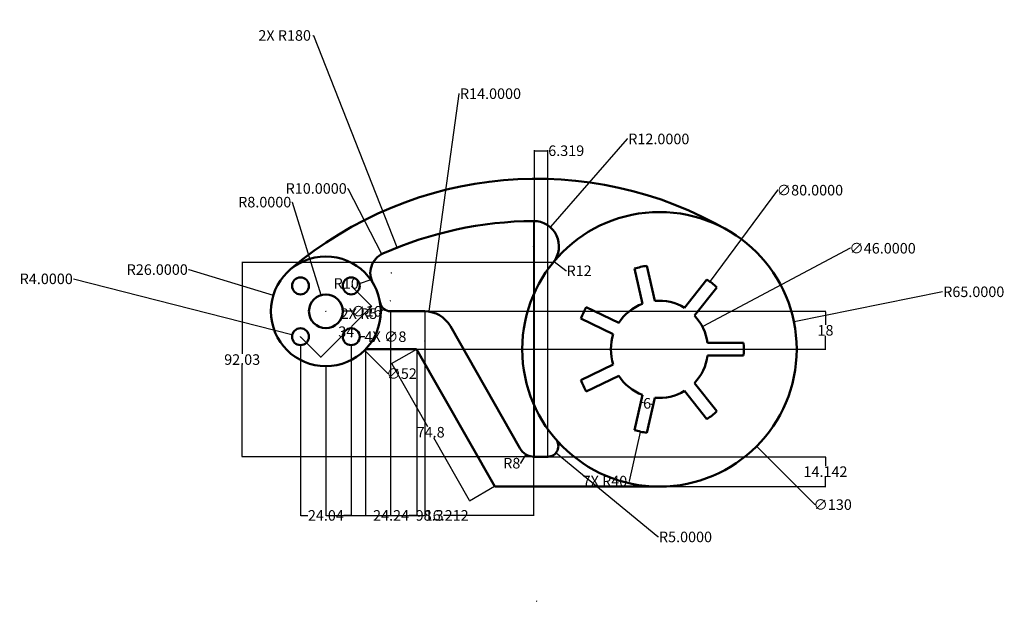
# Model space of a CAD drawing. Units: inches. Extents: x 1057 to 1523, y 448 to 723.
import ezdxf

# ---------------------------------------------------------------- set-up
doc = ezdxf.new("R2010")
doc.units = ezdxf.units.IN
doc.header["$MEASUREMENT"] = 0
doc.layers.add('M-DIMS', color=2, linetype='Continuous', lineweight=25)
doc.layers.add('M-OUTL', color=241, linetype='Continuous', lineweight=50)
doc.styles.get("Standard").update_dxf_attribs({"font": 'arial.ttf'})
doc.dimstyles.get("Standard").update_dxf_attribs({"dimtxt": 5, "dimasz": 0.18, "dimexe": 0.18, "dimexo": 0.0625, "dimgap": 0.09, "dimtad": 0, "dimtih": 1, "dimtoh": 1, "dimdec": 4, "dimzin": 0, "dimdsep": 46, "dimtxsty": 'Standard', "dimcen": 0.09, "dimadec": 0, "dimazin": 0, "dimtfac": 1, "dimtdec": 4, "dimtofl": 0, "dimtmove": 0, "dimatfit": 3, "dimfxl": 1, "dimtolj": 1, "dimtzin": 0, "dimarcsym": 0})

# ---------------------------------------------------------------- blocks, each defined once
blk = doc.blocks.new('*D1')
at = {"layer": 'Defpoints', "color": 0, "transparency": 16777216}
for p in [(1185.77, 574.21), (1189.65, 573.23)]:
    blk.add_point(p, dxfattribs=at)
at = {"layer": 'M-DIMS', "color": 0, "lineweight": -2, "transparency": 16777216}
for p, q in [((1082.06, 600.62), (1185.6, 574.26)), ((1189.56, 573.23), (1189.74, 573.23)), ((1189.65, 573.14), (1189.65, 573.32))]:
    blk.add_line(p, q, dxfattribs=at)
at = {"layer": 'M-DIMS', "color": 0, "transparency": 16777216}
blk.add_solid([(1185.6, 574.29), (1185.59, 574.23), (1185.77, 574.21)], dxfattribs=at)
at = {"layer": 'M-DIMS', "color": 0, "transparency": 16777216, "insert": (1069.21, 600.62), "char_height": 5, "attachment_point": 5}
blk.add_mtext('\\A1;R4.0000', dxfattribs=at)
blk = doc.blocks.new('*D2')
at = {"layer": 'Defpoints', "color": 0, "transparency": 16777216}
for p in [(1176.79, 592.82), (1201.67, 585.25)]:
    blk.add_point(p, dxfattribs=at)
at = {"layer": 'M-DIMS', "color": 0, "lineweight": -2, "transparency": 16777216}
for p, q in [((1136.58, 605), (1136.76, 605)), ((1136.76, 605), (1176.62, 592.87)), ((1201.58, 585.25), (1201.76, 585.25)), ((1201.67, 585.16), (1201.67, 585.34))]:
    blk.add_line(p, q, dxfattribs=at)
at = {"layer": 'M-DIMS', "color": 0, "transparency": 16777216}
blk.add_solid([(1176.63, 592.9), (1176.61, 592.84), (1176.79, 592.82)], dxfattribs=at)
at = {"layer": 'M-DIMS', "color": 0, "transparency": 16777216, "insert": (1121.78, 605), "char_height": 5, "attachment_point": 5}
blk.add_mtext('\\A1;R26.0000', dxfattribs=at)
blk = doc.blocks.new('*D3')
at = {"layer": 'Defpoints', "color": 0, "transparency": 16777216}
for p in [(1199.31, 592.89), (1201.67, 585.25)]:
    blk.add_point(p, dxfattribs=at)
at = {"layer": 'M-DIMS', "color": 0, "lineweight": -2, "transparency": 16777216}
for p, q in [((1185.55, 636.95), (1185.73, 636.95)), ((1185.73, 636.95), (1199.26, 593.07)), ((1201.58, 585.25), (1201.76, 585.25)), ((1201.67, 585.16), (1201.67, 585.34))]:
    blk.add_line(p, q, dxfattribs=at)
at = {"layer": 'M-DIMS', "color": 0, "transparency": 16777216}
blk.add_solid([(1199.29, 593.07), (1199.23, 593.06), (1199.31, 592.89)], dxfattribs=at)
at = {"layer": 'M-DIMS', "color": 0, "transparency": 16777216, "insert": (1172.7, 636.95), "char_height": 5, "attachment_point": 5}
blk.add_mtext('\\A1;R8.0000', dxfattribs=at)
blk = doc.blocks.new('*D4')
at = {"layer": 'Defpoints', "color": 0, "transparency": 16777216}
for p in [(1423.37, 580.19), (1359.67, 567.25)]:
    blk.add_point(p, dxfattribs=at)
at = {"layer": 'M-DIMS', "color": 0, "lineweight": -2, "transparency": 16777216}
for p, q in [((1493.75, 594.49), (1423.54, 580.22)), ((1359.58, 567.25), (1359.76, 567.25)), ((1359.67, 567.16), (1359.67, 567.34))]:
    blk.add_line(p, q, dxfattribs=at)
at = {"layer": 'M-DIMS', "color": 0, "transparency": 16777216}
blk.add_solid([(1423.54, 580.25), (1423.55, 580.19), (1423.37, 580.19)], dxfattribs=at)
at = {"layer": 'M-DIMS', "color": 0, "transparency": 16777216, "insert": (1508.55, 594.49), "char_height": 5, "attachment_point": 5}
blk.add_mtext('\\A1;R65.0000', dxfattribs=at)
blk = doc.blocks.new('*D5')
at = {"layer": 'Defpoints', "color": 0, "transparency": 16777216}
for p in [(1383.52, 599.36), (1335.82, 535.14)]:
    blk.add_point(p, dxfattribs=at)
at = {"layer": 'M-DIMS', "color": 0, "lineweight": -2, "transparency": 16777216}
for p, q in [((1415.64, 642.61), (1383.62, 599.51)), ((1415.82, 642.61), (1415.64, 642.61)), ((1359.58, 567.25), (1359.76, 567.25)), ((1359.67, 567.16), (1359.67, 567.34))]:
    blk.add_line(p, q, dxfattribs=at)
at = {"layer": 'M-DIMS', "color": 0, "transparency": 16777216}
blk.add_solid([(1383.6, 599.52), (1383.65, 599.49), (1383.52, 599.36)], dxfattribs=at)
at = {"layer": 'M-DIMS', "color": 0, "transparency": 16777216, "insert": (1430.94, 642.61), "char_height": 5, "attachment_point": 5}
blk.add_mtext('\\A1;∅80.0000', dxfattribs=at)
blk = doc.blocks.new('*D6')
at = {"layer": 'Defpoints', "color": 0, "transparency": 16777216}
for p in [(1379.99, 578.01), (1339.34, 556.48)]:
    blk.add_point(p, dxfattribs=at)
at = {"layer": 'M-DIMS', "color": 0, "lineweight": -2, "transparency": 16777216}
for p, q in [((1450.04, 615.11), (1380.15, 578.1)), ((1450.22, 615.11), (1450.04, 615.11)), ((1359.58, 567.25), (1359.76, 567.25)), ((1359.67, 567.16), (1359.67, 567.34))]:
    blk.add_line(p, q, dxfattribs=at)
at = {"layer": 'M-DIMS', "color": 0, "transparency": 16777216}
blk.add_solid([(1380.14, 578.12), (1380.17, 578.07), (1379.99, 578.01)], dxfattribs=at)
at = {"layer": 'M-DIMS', "color": 0, "transparency": 16777216, "insert": (1465.34, 615.11), "char_height": 5, "attachment_point": 5}
blk.add_mtext('\\A1;∅46.0000', dxfattribs=at)
blk = doc.blocks.new('*D7')
at = {"layer": 'Defpoints', "color": 0, "transparency": 16777216}
for p in [(1307.96, 625.06), (1300.08, 616.02)]:
    blk.add_point(p, dxfattribs=at)
at = {"layer": 'M-DIMS', "color": 0, "lineweight": -2, "transparency": 16777216}
for p, q in [((1344.4, 666.88), (1308.08, 625.2)), ((1344.58, 666.88), (1344.4, 666.88)), ((1299.99, 616.02), (1300.17, 616.02)), ((1300.08, 615.93), (1300.08, 616.11))]:
    blk.add_line(p, q, dxfattribs=at)
at = {"layer": 'M-DIMS', "color": 0, "transparency": 16777216}
blk.add_solid([(1308.06, 625.22), (1308.1, 625.18), (1307.96, 625.06)], dxfattribs=at)
at = {"layer": 'M-DIMS', "color": 0, "transparency": 16777216, "insert": (1359.37, 666.88), "char_height": 5, "attachment_point": 5}
blk.add_mtext('\\A1;R12.0000', dxfattribs=at)
blk = doc.blocks.new('*D8')
at = {"layer": 'Defpoints', "color": 0, "transparency": 16777216}
for p in [(1306.78, 521.39), (1310.64, 518.21)]:
    blk.add_point(p, dxfattribs=at)
at = {"layer": 'M-DIMS', "color": 0, "lineweight": -2, "transparency": 16777216}
for p, q in [((1306.69, 521.39), (1306.87, 521.39)), ((1306.78, 521.3), (1306.78, 521.48)), ((1358.97, 478.42), (1310.78, 518.1)), ((1359.15, 478.42), (1358.97, 478.42))]:
    blk.add_line(p, q, dxfattribs=at)
at = {"layer": 'M-DIMS', "color": 0, "transparency": 16777216}
blk.add_solid([(1310.8, 518.12), (1310.76, 518.07), (1310.64, 518.21)], dxfattribs=at)
at = {"layer": 'M-DIMS', "color": 0, "transparency": 16777216, "insert": (1372, 478.42), "char_height": 5, "attachment_point": 5}
blk.add_mtext('\\A1;R5.0000', dxfattribs=at)
blk = doc.blocks.new('*D9')
at = {"layer": 'Defpoints', "color": 0, "transparency": 16777216}
for p in [(1228.12, 612.35), (1232.72, 603.47)]:
    blk.add_point(p, dxfattribs=at)
at = {"layer": 'M-DIMS', "color": 0, "lineweight": -2, "transparency": 16777216}
for p, q in [((1211.86, 643.42), (1212.04, 643.42)), ((1212.04, 643.42), (1228.04, 612.51)), ((1232.63, 603.47), (1232.81, 603.47)), ((1232.72, 603.38), (1232.72, 603.56))]:
    blk.add_line(p, q, dxfattribs=at)
at = {"layer": 'M-DIMS', "color": 0, "transparency": 16777216}
blk.add_solid([(1228.06, 612.52), (1228.01, 612.5), (1228.12, 612.35)], dxfattribs=at)
at = {"layer": 'M-DIMS', "color": 0, "transparency": 16777216, "insert": (1197.07, 643.42), "char_height": 5, "attachment_point": 5}
blk.add_mtext('\\A1;R10.0000', dxfattribs=at)
blk = doc.blocks.new('*D10')
at = {"layer": 'Defpoints', "color": 0, "transparency": 16777216}
for p in [(1250.39, 585.12), (1248.47, 571.25)]:
    blk.add_point(p, dxfattribs=at)
at = {"layer": 'M-DIMS', "color": 0, "lineweight": -2, "transparency": 16777216}
for p, q in [((1264.66, 688.31), (1250.42, 585.29)), ((1264.84, 688.31), (1264.66, 688.31)), ((1248.38, 571.25), (1248.56, 571.25)), ((1248.47, 571.16), (1248.47, 571.34))]:
    blk.add_line(p, q, dxfattribs=at)
at = {"layer": 'M-DIMS', "color": 0, "transparency": 16777216}
blk.add_solid([(1250.39, 585.3), (1250.45, 585.29), (1250.39, 585.12)], dxfattribs=at)
at = {"layer": 'M-DIMS', "color": 0, "transparency": 16777216, "insert": (1279.63, 688.31), "char_height": 5, "attachment_point": 5}
blk.add_mtext('\\A1;R14.0000', dxfattribs=at)
blk = doc.blocks.new('PIVOT-MOUNT-HOLE-D8')
blk.add_circle((4, 4), 4)
blk = doc.blocks.new('*D12')
at = {"layer": 'Defpoints', "color": 0, "transparency": 16777216}
for p in [(1299.98, 628.02), (1201.67, 559.25), (1299.98, 488.6)]:
    blk.add_point(p, dxfattribs=at)
at = {"layer": 'M-DIMS', "color": 0, "lineweight": -2, "transparency": 16777216}
for p, q in [((1299.98, 627.95), (1299.98, 488.42)), ((1201.67, 559.19), (1201.67, 488.42)), ((1201.85, 488.6), (1244.24, 488.6)), ((1299.8, 488.6), (1257.41, 488.6))]:
    blk.add_line(p, q, dxfattribs=at)
at = {"layer": 'M-DIMS', "color": 0, "transparency": 16777216}
for points in [[(1201.85, 488.63), (1201.85, 488.57), (1201.67, 488.6)], [(1299.8, 488.63), (1299.8, 488.57), (1299.98, 488.6)]]:
    blk.add_solid(points, dxfattribs=at)
at = {"layer": 'M-DIMS', "color": 0, "transparency": 16777216, "insert": (1250.82, 488.6), "char_height": 5, "attachment_point": 5}
blk.add_mtext('\\A1;98.3', dxfattribs=at)
blk = doc.blocks.new('*D13')
at = {"layer": 'Defpoints', "color": 0, "transparency": 16777216}
for p in [(1309.37, 608.42), (1162.02, 516.39), (1306.78, 516.39)]:
    blk.add_point(p, dxfattribs=at)
at = {"layer": 'M-DIMS', "color": 0, "lineweight": -2, "transparency": 16777216}
for p, q in [((1309.3, 608.42), (1161.84, 608.42)), ((1162.02, 608.24), (1162.02, 565.05)), ((1162.02, 516.57), (1162.02, 559.76)), ((1306.72, 516.39), (1161.84, 516.39))]:
    blk.add_line(p, q, dxfattribs=at)
at = {"layer": 'M-DIMS', "color": 0, "transparency": 16777216}
for points in [[(1161.99, 608.24), (1162.05, 608.24), (1162.02, 608.42)], [(1161.99, 516.57), (1162.05, 516.57), (1162.02, 516.39)]]:
    blk.add_solid(points, dxfattribs=at)
at = {"layer": 'M-DIMS', "color": 0, "transparency": 16777216, "insert": (1162.02, 562.4), "char_height": 5, "attachment_point": 5}
blk.add_mtext('\\A1;92.03', dxfattribs=at)
blk = doc.blocks.new('*D14')
at = {"layer": 'Defpoints', "color": 0, "transparency": 16777216}
for p in [(1248.47, 585.25), (1244.67, 567.25), (1438.32, 567.25)]:
    blk.add_point(p, dxfattribs=at)
at = {"layer": 'M-DIMS', "color": 0, "lineweight": -2, "transparency": 16777216}
for p, q in [((1248.54, 585.25), (1438.5, 585.25)), ((1438.32, 585.07), (1438.32, 578.89)), ((1438.32, 567.43), (1438.32, 573.61)), ((1244.73, 567.25), (1438.5, 567.25))]:
    blk.add_line(p, q, dxfattribs=at)
at = {"layer": 'M-DIMS', "color": 0, "transparency": 16777216}
for points in [[(1438.29, 585.07), (1438.35, 585.07), (1438.32, 585.25)], [(1438.29, 567.43), (1438.35, 567.43), (1438.32, 567.25)]]:
    blk.add_solid(points, dxfattribs=at)
at = {"layer": 'M-DIMS', "color": 0, "transparency": 16777216, "insert": (1438.32, 576.25), "char_height": 5, "attachment_point": 5}
blk.add_mtext('\\A1;18', dxfattribs=at)
blk = doc.blocks.new('*D15')
at = {"layer": 'Defpoints', "color": 0, "transparency": 16777216}
for p in [(1220.43, 567.25), (1244.67, 567.25), (1244.67, 488.6)]:
    blk.add_point(p, dxfattribs=at)
at = {"layer": 'M-DIMS', "color": 0, "lineweight": -2, "transparency": 16777216}
for p, q in [((1220.43, 567.19), (1220.43, 488.42)), ((1244.67, 567.19), (1244.67, 488.42)), ((1220.61, 488.6), (1223.99, 488.6)), ((1244.49, 488.6), (1241.11, 488.6))]:
    blk.add_line(p, q, dxfattribs=at)
at = {"layer": 'M-DIMS', "color": 0, "transparency": 16777216}
for points in [[(1220.61, 488.63), (1220.61, 488.57), (1220.43, 488.6)], [(1244.49, 488.63), (1244.49, 488.57), (1244.67, 488.6)]]:
    blk.add_solid(points, dxfattribs=at)
at = {"layer": 'M-DIMS', "color": 0, "transparency": 16777216, "insert": (1232.55, 488.6), "char_height": 5, "attachment_point": 5}
blk.add_mtext('\\A1;24.24', dxfattribs=at)
blk = doc.blocks.new('*D16')
at = {"layer": 'Defpoints', "color": 0, "transparency": 16777216}
for p in [(1244.67, 567.25), (1232.81, 560.5), (1281.67, 502.25)]:
    blk.add_point(p, dxfattribs=at)
at = {"layer": 'M-DIMS', "color": 0, "lineweight": -2, "transparency": 16777216}
for p, q in [((1244.61, 567.22), (1232.65, 560.41)), ((1232.89, 560.34), (1249.8, 530.64)), ((1269.72, 495.65), (1252.81, 525.35)), ((1281.61, 502.22), (1269.65, 495.41))]:
    blk.add_line(p, q, dxfattribs=at)
at = {"layer": 'M-DIMS', "color": 0, "transparency": 16777216}
for points in [[(1232.92, 560.35), (1232.87, 560.32), (1232.81, 560.5)], [(1269.74, 495.67), (1269.69, 495.64), (1269.81, 495.5)]]:
    blk.add_solid(points, dxfattribs=at)
at = {"layer": 'M-DIMS', "color": 0, "transparency": 16777216, "insert": (1251.31, 528), "char_height": 5, "attachment_point": 5}
blk.add_mtext('\\A1;74.8', dxfattribs=at)
blk = doc.blocks.new('*D17')
at = {"layer": 'Defpoints', "color": 0, "transparency": 16777216}
for p in [(1300.46, 516.39), (1438.32, 516.39), (1281.67, 502.25)]:
    blk.add_point(p, dxfattribs=at)
at = {"layer": 'M-DIMS', "color": 0, "lineweight": -2, "transparency": 16777216}
for p, q in [((1300.52, 516.39), (1438.5, 516.39)), ((1438.32, 516.21), (1438.32, 511.92)), ((1438.32, 502.43), (1438.32, 506.72)), ((1281.73, 502.25), (1438.5, 502.25))]:
    blk.add_line(p, q, dxfattribs=at)
at = {"layer": 'M-DIMS', "color": 0, "transparency": 16777216}
for points in [[(1438.29, 516.21), (1438.35, 516.21), (1438.32, 516.39)], [(1438.29, 502.43), (1438.35, 502.43), (1438.32, 502.25)]]:
    blk.add_solid(points, dxfattribs=at)
at = {"layer": 'M-DIMS', "color": 0, "transparency": 16777216, "insert": (1438.32, 509.32), "char_height": 5, "attachment_point": 5}
blk.add_mtext('\\A1;14.142', dxfattribs=at)
blk = doc.blocks.new('*D18')
at = {"layer": 'Defpoints', "color": 0, "transparency": 16777216}
for p in [(1213.69, 597.27), (1189.65, 573.23), (1199.3, 563.58)]:
    blk.add_point(p, dxfattribs=at)
at = {"layer": 'M-DIMS', "color": 0, "lineweight": -2, "transparency": 16777216}
for p, q in [((1213.73, 597.23), (1223.47, 587.49)), ((1223.21, 587.49), (1213.96, 578.24)), ((1189.69, 573.18), (1199.43, 563.45)), ((1199.43, 563.7), (1208.68, 572.95))]:
    blk.add_line(p, q, dxfattribs=at)
at = {"layer": 'M-DIMS', "color": 0, "transparency": 16777216}
for points in [[(1223.19, 587.51), (1223.23, 587.47), (1223.34, 587.62)], [(1199.41, 563.72), (1199.45, 563.68), (1199.3, 563.58)]]:
    blk.add_solid(points, dxfattribs=at)
at = {"layer": 'M-DIMS', "color": 0, "transparency": 16777216, "insert": (1211.32, 575.6), "char_height": 5, "attachment_point": 5}
blk.add_mtext('\\A1;34', dxfattribs=at)
blk = doc.blocks.new('*D19')
at = {"layer": 'Defpoints', "color": 0, "transparency": 16777216}
for p in [(1189.65, 569.23), (1213.69, 569.23), (1213.69, 488.6)]:
    blk.add_point(p, dxfattribs=at)
at = {"layer": 'M-DIMS', "color": 0, "lineweight": -2, "transparency": 16777216}
for p, q in [((1189.65, 569.17), (1189.65, 488.42)), ((1213.69, 569.17), (1213.69, 488.42)), ((1189.83, 488.6), (1193.11, 488.6)), ((1213.51, 488.6), (1210.23, 488.6))]:
    blk.add_line(p, q, dxfattribs=at)
at = {"layer": 'M-DIMS', "color": 0, "transparency": 16777216}
for points in [[(1189.83, 488.63), (1189.83, 488.57), (1189.65, 488.6)], [(1213.51, 488.63), (1213.51, 488.57), (1213.69, 488.6)]]:
    blk.add_solid(points, dxfattribs=at)
at = {"layer": 'M-DIMS', "color": 0, "transparency": 16777216, "insert": (1201.67, 488.6), "char_height": 5, "attachment_point": 5}
blk.add_mtext('\\A1;24.04', dxfattribs=at)
blk = doc.blocks.new('*D20')
at = {"layer": 'Defpoints', "color": 0, "transparency": 16777216}
for p in [(1356.75, 541), (1347.87, 529.03), (1353.72, 527.69)]:
    blk.add_point(p, dxfattribs=at)
at = {"layer": 'M-DIMS', "color": 0, "lineweight": -2, "transparency": 16777216}
for p, q in [((1347.88, 529.09), (1350.94, 542.51)), ((1351.08, 542.3), (1352.09, 542.07)), ((1353.73, 527.75), (1356.79, 541.18)), ((1356.58, 541.04), (1355.57, 541.27))]:
    blk.add_line(p, q, dxfattribs=at)
at = {"layer": 'M-DIMS', "color": 0, "transparency": 16777216}
for points in [[(1351.09, 542.33), (1351.07, 542.27), (1350.9, 542.34)], [(1356.59, 541.07), (1356.57, 541.01), (1356.75, 541)]]:
    blk.add_solid(points, dxfattribs=at)
at = {"layer": 'M-DIMS', "color": 0, "transparency": 16777216, "insert": (1353.83, 541.67), "char_height": 5, "attachment_point": 5}
blk.add_mtext('\\A1;6', dxfattribs=at)
blk = doc.blocks.new('*D21')
at = {"layer": 'Defpoints', "color": 0, "transparency": 16777216}
for p in [(1232.26, 585.25), (1248.47, 585.25), (1248.47, 488.6)]:
    blk.add_point(p, dxfattribs=at)
at = {"layer": 'M-DIMS', "color": 0, "lineweight": -2, "transparency": 16777216}
for p, q in [((1232.26, 585.19), (1232.26, 488.42)), ((1248.47, 585.19), (1248.47, 488.42)), ((1232.44, 488.6), (1248.29, 488.6)), ((1248.47, 488.6), (1248.65, 488.6))]:
    blk.add_line(p, q, dxfattribs=at)
at = {"layer": 'M-DIMS', "color": 0, "transparency": 16777216}
for points in [[(1232.44, 488.63), (1232.44, 488.57), (1232.26, 488.6)], [(1248.29, 488.63), (1248.29, 488.57), (1248.47, 488.6)]]:
    blk.add_solid(points, dxfattribs=at)
at = {"layer": 'M-DIMS', "color": 0, "transparency": 16777216, "insert": (1258.86, 488.6), "char_height": 5, "attachment_point": 5}
blk.add_mtext('\\A1;16.212', dxfattribs=at)
blk = doc.blocks.new('*D22')
at = {"layer": 'Defpoints', "color": 0, "transparency": 16777216}
for p in [(1306.78, 661.3), (1300.46, 516.39), (1306.78, 516.39)]:
    blk.add_point(p, dxfattribs=at)
at = {"layer": 'M-DIMS', "color": 0, "lineweight": -2, "transparency": 16777216}
for p, q in [((1300.46, 516.45), (1300.46, 661.48)), ((1300.64, 661.3), (1306.6, 661.3)), ((1306.78, 516.45), (1306.78, 661.48)), ((1306.78, 661.3), (1306.96, 661.3))]:
    blk.add_line(p, q, dxfattribs=at)
at = {"layer": 'M-DIMS', "color": 0, "transparency": 16777216}
for points in [[(1300.64, 661.33), (1300.64, 661.27), (1300.46, 661.3)], [(1306.6, 661.33), (1306.6, 661.27), (1306.78, 661.3)]]:
    blk.add_solid(points, dxfattribs=at)
at = {"layer": 'M-DIMS', "color": 0, "transparency": 16777216, "insert": (1315.51, 661.3), "char_height": 5, "attachment_point": 5}
blk.add_mtext('\\A1;6.319', dxfattribs=at)
blk = doc.blocks.new('*D23')
at = {"layer": 'Defpoints', "color": 0, "transparency": 16777216}
for p in [(1235.41, 615.43), (1301.54, 448.02)]:
    blk.add_point(p, dxfattribs=at)
at = {"layer": 'M-DIMS', "color": 0, "lineweight": -2, "transparency": 16777216}
for p, q in [((1195.55, 715.88), (1195.73, 715.88)), ((1195.73, 715.88), (1235.34, 615.6)), ((1301.45, 448.02), (1301.63, 448.02)), ((1301.54, 447.93), (1301.54, 448.11))]:
    blk.add_line(p, q, dxfattribs=at)
at = {"layer": 'M-DIMS', "color": 0, "transparency": 16777216}
blk.add_solid([(1235.37, 615.61), (1235.31, 615.59), (1235.41, 615.43)], dxfattribs=at)
at = {"layer": 'M-DIMS', "color": 0, "transparency": 16777216, "insert": (1182.14, 715.88), "char_height": 5, "attachment_point": 5}
blk.add_mtext('\\A1;2X R180', dxfattribs=at)
blk = doc.blocks.new('*D24')
at = {"layer": 'Defpoints', "color": 0, "transparency": 16777216}
for p in [(1313.7, 613.21), (1405.63, 521.29)]:
    blk.add_point(p, dxfattribs=at)
at = {"layer": 'M-DIMS', "color": 0, "lineweight": -2, "transparency": 16777216}
for p, q in [((1359.58, 567.25), (1359.76, 567.25)), ((1359.67, 567.16), (1359.67, 567.34)), ((1433.21, 493.71), (1405.76, 521.16)), ((1433.39, 493.71), (1433.21, 493.71))]:
    blk.add_line(p, q, dxfattribs=at)
at = {"layer": 'M-DIMS', "color": 0, "transparency": 16777216}
blk.add_solid([(1405.78, 521.18), (1405.74, 521.14), (1405.63, 521.29)], dxfattribs=at)
at = {"layer": 'M-DIMS', "color": 0, "transparency": 16777216, "insert": (1441.71, 493.71), "char_height": 5, "attachment_point": 5}
blk.add_mtext('\\A1;∅130', dxfattribs=at)
blk = doc.blocks.new('*D25')
at = {"layer": 'Defpoints', "color": 0, "transparency": 16777216}
for p in [(1359.67, 567.25), (1350.77, 528.25)]:
    blk.add_point(p, dxfattribs=at)
at = {"layer": 'M-DIMS', "color": 0, "lineweight": -2, "transparency": 16777216}
for p, q in [((1359.58, 567.25), (1359.76, 567.25)), ((1359.67, 567.16), (1359.67, 567.34)), ((1345.43, 504.85), (1350.73, 528.08)), ((1345.25, 504.85), (1345.43, 504.85))]:
    blk.add_line(p, q, dxfattribs=at)
at = {"layer": 'M-DIMS', "color": 0, "transparency": 16777216}
blk.add_solid([(1350.7, 528.08), (1350.76, 528.07), (1350.77, 528.25)], dxfattribs=at)
at = {"layer": 'M-DIMS', "color": 0, "transparency": 16777216, "insert": (1333.84, 504.85), "char_height": 5, "attachment_point": 5}
blk.add_mtext('\\A1;7X R40', dxfattribs=at)
blk = doc.blocks.new('*D26')
at = {"layer": 'Defpoints', "color": 0, "transparency": 16777216}
for p in [(1183.34, 603.69), (1219.99, 566.81)]:
    blk.add_point(p, dxfattribs=at)
at = {"layer": 'M-DIMS', "color": 0, "lineweight": -2, "transparency": 16777216}
for p, q in [((1201.58, 585.25), (1201.76, 585.25)), ((1201.67, 585.16), (1201.67, 585.34)), ((1230.99, 555.74), (1220.12, 566.68)), ((1231.17, 555.74), (1230.99, 555.74))]:
    blk.add_line(p, q, dxfattribs=at)
at = {"layer": 'M-DIMS', "color": 0, "transparency": 16777216}
blk.add_solid([(1220.14, 566.7), (1220.1, 566.66), (1219.99, 566.81)], dxfattribs=at)
at = {"layer": 'M-DIMS', "color": 0, "transparency": 16777216, "insert": (1237.54, 555.74), "char_height": 5, "attachment_point": 5}
blk.add_mtext('\\A1;∅52', dxfattribs=at)
blk = doc.blocks.new('*D27')
at = {"layer": 'Defpoints', "color": 0, "transparency": 16777216}
for p in [(1300.08, 616.02), (1309.65, 608.78)]:
    blk.add_point(p, dxfattribs=at)
at = {"layer": 'M-DIMS', "color": 0, "lineweight": -2, "transparency": 16777216}
for p, q in [((1299.99, 616.02), (1300.17, 616.02)), ((1300.08, 615.93), (1300.08, 616.11)), ((1315.4, 604.44), (1309.8, 608.67)), ((1315.58, 604.44), (1315.4, 604.44))]:
    blk.add_line(p, q, dxfattribs=at)
at = {"layer": 'M-DIMS', "color": 0, "transparency": 16777216}
blk.add_solid([(1309.82, 608.7), (1309.78, 608.65), (1309.65, 608.78)], dxfattribs=at)
at = {"layer": 'M-DIMS', "color": 0, "transparency": 16777216, "insert": (1321.62, 604.44), "char_height": 5, "attachment_point": 5}
blk.add_mtext('\\A1;R12', dxfattribs=at)
blk = doc.blocks.new('*D28')
at = {"layer": 'Defpoints', "color": 0, "transparency": 16777216}
for p in [(1232.72, 603.47), (1223.23, 600.32)]:
    blk.add_point(p, dxfattribs=at)
at = {"layer": 'M-DIMS', "color": 0, "lineweight": -2, "transparency": 16777216}
for p, q in [((1232.63, 603.47), (1232.81, 603.47)), ((1232.72, 603.38), (1232.72, 603.56)), ((1217.35, 598.42), (1217.53, 598.42)), ((1217.53, 598.42), (1223.06, 600.26))]:
    blk.add_line(p, q, dxfattribs=at)
at = {"layer": 'M-DIMS', "color": 0, "transparency": 16777216}
blk.add_solid([(1223.05, 600.29), (1223.07, 600.23), (1223.23, 600.32)], dxfattribs=at)
at = {"layer": 'M-DIMS', "color": 0, "transparency": 16777216, "insert": (1211.3, 598.42), "char_height": 5, "attachment_point": 5}
blk.add_mtext('\\A1;R10', dxfattribs=at)
blk = doc.blocks.new('*D29')
at = {"layer": 'Defpoints', "color": 0, "transparency": 16777216}
for p in [(1193.67, 585.25), (1209.67, 585.25)]:
    blk.add_point(p, dxfattribs=at)
at = {"layer": 'M-DIMS', "color": 0, "lineweight": -2, "transparency": 16777216}
for p, q in [((1201.58, 585.25), (1201.76, 585.25)), ((1201.67, 585.16), (1201.67, 585.34)), ((1214.47, 585.25), (1209.85, 585.25))]:
    blk.add_line(p, q, dxfattribs=at)
at = {"layer": 'M-DIMS', "color": 0, "transparency": 16777216}
blk.add_solid([(1209.85, 585.28), (1209.85, 585.22), (1209.67, 585.25)], dxfattribs=at)
at = {"layer": 'M-DIMS', "color": 0, "transparency": 16777216, "insert": (1220.86, 585.25), "char_height": 5, "attachment_point": 5}
blk.add_mtext('\\A1;∅16', dxfattribs=at)
blk = doc.blocks.new('*D30')
at = {"layer": 'Defpoints', "color": 0, "transparency": 16777216}
for p in [(1300.46, 524.39), (1296.44, 517.47)]:
    blk.add_point(p, dxfattribs=at)
at = {"layer": 'M-DIMS', "color": 0, "lineweight": -2, "transparency": 16777216}
for p, q in [((1300.37, 524.39), (1300.55, 524.39)), ((1300.46, 524.3), (1300.46, 524.48)), ((1293.85, 513.33), (1294.03, 513.33)), ((1294.03, 513.33), (1296.35, 517.32))]:
    blk.add_line(p, q, dxfattribs=at)
at = {"layer": 'M-DIMS', "color": 0, "transparency": 16777216}
blk.add_solid([(1296.32, 517.33), (1296.38, 517.3), (1296.44, 517.47)], dxfattribs=at)
at = {"layer": 'M-DIMS', "color": 0, "transparency": 16777216, "insert": (1289.72, 513.33), "char_height": 5, "attachment_point": 5}
blk.add_mtext('\\A1;R8', dxfattribs=at)
blk = doc.blocks.new('*D31')
at = {"layer": 'Defpoints', "color": 0, "transparency": 16777216}
for p in [(1232.26, 590.25), (1229.02, 586.44)]:
    blk.add_point(p, dxfattribs=at)
at = {"layer": 'M-DIMS', "color": 0, "lineweight": -2, "transparency": 16777216}
for p, q in [((1232.17, 590.25), (1232.35, 590.25)), ((1232.26, 590.16), (1232.26, 590.34)), ((1226.9, 584.15), (1227.08, 584.15)), ((1227.08, 584.15), (1228.91, 586.3))]:
    blk.add_line(p, q, dxfattribs=at)
at = {"layer": 'M-DIMS', "color": 0, "transparency": 16777216}
blk.add_solid([(1228.88, 586.32), (1228.93, 586.28), (1229.02, 586.44)], dxfattribs=at)
at = {"layer": 'M-DIMS', "color": 0, "transparency": 16777216, "insert": (1217.35, 584.15), "char_height": 5, "attachment_point": 5}
blk.add_mtext('\\A1;2X R5', dxfattribs=at)
blk = doc.blocks.new('*D32')
at = {"layer": 'Defpoints', "color": 0, "transparency": 16777216}
for p in [(1209.69, 573.23), (1217.69, 573.23)]:
    blk.add_point(p, dxfattribs=at)
at = {"layer": 'M-DIMS', "color": 0, "lineweight": -2, "transparency": 16777216}
for p, q in [((1213.6, 573.23), (1213.78, 573.23)), ((1213.69, 573.14), (1213.69, 573.32)), ((1220.09, 573.23), (1217.87, 573.23))]:
    blk.add_line(p, q, dxfattribs=at)
at = {"layer": 'M-DIMS', "color": 0, "transparency": 16777216}
blk.add_solid([(1217.87, 573.26), (1217.87, 573.2), (1217.69, 573.23)], dxfattribs=at)
at = {"layer": 'M-DIMS', "color": 0, "transparency": 16777216, "insert": (1229.88, 573.23), "char_height": 5, "attachment_point": 5}
blk.add_mtext('\\A1;4X ∅8', dxfattribs=at)

msp = doc.modelspace()

# ---------------------------------------------------------------- linework, layer by layer
at = {"layer": 'M-OUTL'}
for p, q in [((1357.51835, 590.14784), (1353.71684, 606.80335)), ((1351.66879, 588.81272), (1347.86728, 605.46822)), ((1371.54009, 586.94747), (1382.19168, 600.30415)), ((1376.23108, 583.20654), (1386.88267, 596.56321)), ((1232.26194, 585.2485), (1248.47391, 585.2485)), ((1340.42423, 579.84548), (1325.03223, 587.25788)), ((1337.82093, 574.43967), (1322.42892, 581.85207)), ((1260.64081, 578.17428), (1293.5089, 520.43305)), ((1382.47134, 570.2485), (1399.55517, 570.2485)), ((1220.42949, 567.2485), (1244.66783, 567.2485)), ((1244.66783, 567.2485), (1281.66783, 502.2485)), ((1337.82093, 560.05734), (1322.42892, 552.64494)), ((1382.47134, 564.2485), (1399.55517, 564.2485)), ((1340.42423, 554.65153), (1325.03223, 547.23913)), ((1376.23108, 551.29047), (1386.88267, 537.93379)), ((1351.66879, 545.68429), (1347.86728, 529.02878)), ((1371.54009, 547.54953), (1382.19168, 534.19286)), ((1357.51835, 544.34916), (1353.71684, 527.69366)), ((1300.46142, 516.39064), (1306.78062, 516.39064)), ((1359.66783, 502.2485), (1281.66783, 502.2485))]:
    msp.add_line(p, q, dxfattribs=at)
for centre, radius in [((1359.66783, 567.2485), 65), ((1201.66783, 585.2485), 26), ((1201.66783, 585.2485), 8)]:
    msp.add_circle(centre, radius, dxfattribs=at)
for centre, radius, start, end in [((1301.53761, 468.02211), 180, 59.6367662, 130.4289837), ((1301.53761, 448.02211), 180, 90.497241, 113.880463), ((1300.07964, 616.01578), 12, 320.7029306, 90.497241), ((1232.71654, 603.46876), 10, 113.880463, 210.4056075), ((1359.66783, 567.2485), 40, 98.5559206, 107.1583652), ((1359.66783, 567.2485), 40, 47.1273491, 55.7297937), ((1232.26194, 590.2485), 5, 189.2817991, 270), ((1359.66783, 567.2485), 23, 110.3518603, 146.7909968), ((1359.66783, 567.2485), 23, 58.9232889, 95.3624254), ((1248.47391, 571.2485), 14, 29.6498635, 90), ((1359.66783, 567.2485), 40, 149.984492, 158.5869366), ((1359.66783, 567.2485), 23, 7.4947175, 43.933854), ((1359.66783, 567.2485), 23, 161.7804317, 198.2195683), ((1359.66783, 567.2485), 40, 355.6987777, 4.3012223), ((1359.66783, 567.2485), 23, 316.066146, 352.5052825), ((1359.66783, 567.2485), 40, 201.4130634, 210.015508), ((1359.66783, 567.2485), 23, 213.2090032, 249.6481397), ((1359.66783, 567.2485), 23, 264.6375746, 301.0767111), ((1359.66783, 567.2485), 40, 304.2702063, 312.8726509), ((1359.66783, 567.2485), 40, 252.8416348, 261.4440794), ((1306.78062, 521.39064), 5, 270, 40.9281693), ((1300.46142, 524.39064), 8, 209.6498635, 270)]:
    msp.add_arc(centre, radius, start, end, dxfattribs=at)

# ---------------------------------------------------------------- block references
for p in [(1185.647, 593.269), (1209.68863, 593.269), (1185.647, 569.22737), (1209.68863, 569.22737)]:
    msp.add_blockref('PIVOT-MOUNT-HOLE-D8', p, dxfattribs=at)

# ---------------------------------------------------------------- dimensions: what is measured, and where the dimension line sits
at = {"layer": 'M-DIMS'}
for center, mpoint, text, picture, middle in [((1301.5376, 448.02211), (1235.40767, 615.43427), '2X <>', '*D23', (1182.13774, 715.88157)), ((1232.26194, 590.2485), (1229.02378, 586.43874), '2X <>', '*D31', (1217.34635, 584.15288)), ((1359.66783, 567.2485), (1350.7673, 528.25132), '7X <>', '*D25', (1333.84048, 504.853))]:
    dim = msp.add_radius_dim(center=center, mpoint=mpoint, text=text, dimstyle='Standard', override={"dimdec": 0, "dimlfac": 1, "dimrnd": 0, "dimzin": 0, "dimdsep": 46, "dimlunit": 2}, dxfattribs=at)
    dim.commit()
    dim.dimension.update_dxf_attribs({"geometry": picture, "text_midpoint": middle, "dimtype": 164})
for center, mpoint, override, picture, middle in [((1248.47391, 571.2485), (1250.39138, 585.11657), {"dimclrd": 0, "dimclre": 0, "dimclrt": 0}, '*D10', (1279.63473, 688.31212)), ((1300.07964, 616.01578), (1307.96291, 625.0631), {"dimclrd": 0, "dimclre": 0, "dimclrt": 0}, '*D7', (1359.37258, 666.87776)), ((1232.71654, 603.46876), (1228.12046, 612.34998), {"dimclrd": 0, "dimclre": 0, "dimclrt": 0}, '*D9', (1197.06589, 643.42129)), ((1201.66783, 585.2485), (1199.31135, 592.89357), {"dimclrd": 0, "dimclre": 0, "dimclrt": 0}, '*D3', (1172.69881, 636.95054)), ((1300.07964, 616.01578), (1309.65494, 608.78297), {"dimdec": 0, "dimlfac": 1, "dimrnd": 0, "dimzin": 0, "dimdsep": 46, "dimlunit": 2}, '*D27', (1321.61827, 604.44328)), ((1201.66783, 585.2485), (1176.79396, 592.81757), {"dimclrd": 0, "dimclre": 0, "dimclrt": 0}, '*D2', (1121.78042, 605.00121)), ((1189.64701, 573.22769), (1185.77065, 574.21452), {"dimclrd": 0, "dimclre": 0, "dimclrt": 0}, '*D1', (1082.06197, 600.61643)), ((1232.71654, 603.46876), (1223.22671, 600.31549), {"dimdec": 0, "dimlfac": 1, "dimrnd": 0, "dimzin": 0, "dimdsep": 46, "dimlunit": 2}, '*D28', (1211.2976, 598.42353)), ((1359.66783, 567.2485), (1423.36687, 580.18805), {"dimclrd": 0, "dimclre": 0, "dimclrt": 0}, '*D4', (1493.75427, 594.48624)), ((1300.46141, 524.39064), (1296.43993, 517.47488), {"dimdec": 0, "dimlfac": 1, "dimrnd": 0, "dimzin": 0, "dimdsep": 46, "dimlunit": 2}, '*D30', (1289.72055, 513.32543)), ((1306.78062, 521.39064), (1310.64046, 518.21233), {"dimclrd": 0, "dimclre": 0, "dimclrt": 0}, '*D8', (1372.0016, 478.41716))]:
    dim = msp.add_radius_dim(center=center, mpoint=mpoint, dimstyle='Standard', override=override, dxfattribs=at)
    dim.commit()
    dim.dimension.update_dxf_attribs({"geometry": picture, "text_midpoint": middle, "dimtype": 164})
for base, p1, p2, override, picture, middle in [((1306.78062, 661.30254), (1300.46141, 516.39064), (1306.78062, 516.39064), {"dimdec": 3, "dimlfac": 1, "dimrnd": 0, "dimzin": 0, "dimdsep": 46, "dimlunit": 2}, '*D22', (1315.5056, 661.30254)), ((1299.9755, 488.5985), (1201.66783, 559.2485), (1299.9755, 628.01533), {"dimdec": 1, "dimlfac": 1, "dimrnd": 0, "dimzin": 0, "dimdsep": 46, "dimlunit": 2}, '*D12', (1250.82166, 488.5985)), ((1248.47391, 488.5985), (1232.26194, 585.2485), (1248.47391, 585.2485), {"dimdec": 3, "dimlfac": 1, "dimrnd": 0, "dimzin": 0, "dimdsep": 46, "dimlunit": 2}, '*D21', (1258.86157, 488.5985)), ((1213.68864, 488.5985), (1189.64701, 569.22769), (1213.68864, 569.22769), {"dimdec": 2, "dimlfac": 1, "dimrnd": 0, "dimzin": 0, "dimdsep": 46, "dimlunit": 2}, '*D19', (1201.66783, 488.5985)), ((1244.66783, 488.5985), (1220.42949, 567.2485), (1244.66783, 567.2485), {"dimdec": 2, "dimlfac": 1, "dimrnd": 0, "dimzin": 0, "dimdsep": 46, "dimlunit": 2}, '*D15', (1232.54866, 488.5985))]:
    dim = msp.add_linear_dim(base=base, p1=p1, p2=p2, dimstyle='Standard', override=override, dxfattribs=at)
    dim.commit()
    dim.dimension.update_dxf_attribs({"geometry": picture, "text_midpoint": middle})
for p1, p2, override, picture, middle in [((1335.81954, 535.13528), (1383.51612, 599.36173), {"dimclrd": 0, "dimclre": 0, "dimclrt": 0}, '*D5', (1430.93786, 642.61245)), ((1339.34248, 556.48373), (1379.99317, 578.01328), {"dimclrd": 0, "dimclre": 0, "dimclrt": 0}, '*D6', (1465.34252, 615.11176)), ((1313.70405, 613.20861), (1405.6316, 521.2884), {"dimdec": 0, "dimlfac": 1, "dimrnd": 0, "dimzin": 0, "dimdsep": 46, "dimlunit": 2}, '*D24', (1441.71486, 493.71233)), ((1183.34129, 603.69134), (1219.99436, 566.80567), {"dimdec": 0, "dimlfac": 1, "dimrnd": 0, "dimzin": 0, "dimdsep": 46, "dimlunit": 2}, '*D26', (1237.53587, 555.73997)), ((1193.66783, 585.24801), (1209.66783, 585.249), {"dimdec": 0, "dimlfac": 1, "dimrnd": 0, "dimzin": 0, "dimdsep": 46, "dimlunit": 2}, '*D29', (1214.46783, 585.2493))]:
    dim = msp.add_diameter_dim_2p(p1=p1, p2=p2, dimstyle='Standard', override=override, dxfattribs=at)
    dim.commit()
    dim.dimension.update_dxf_attribs({"geometry": picture, "text_midpoint": middle, "dimtype": 163})
for base, p1, p2, angle, override, picture, middle in [((1162.01783, 516.39064), (1309.36611, 608.41569), (1306.78062, 516.39064), 90, {"dimdec": 2, "dimlfac": 1, "dimrnd": 0, "dimzin": 0, "dimdsep": 46, "dimlunit": 2}, '*D13', (1162.01783, 562.40316)), ((1199.29902, 563.57568), (1213.68864, 597.26932), (1189.64701, 573.22769), 225, {"dimdec": 0, "dimlfac": 1, "dimrnd": 0, "dimzin": 0, "dimdsep": 46, "dimlunit": 2}, '*D18', (1211.31984, 575.5965)), ((1438.31783, 567.2485), (1248.47391, 585.2485), (1244.66783, 567.2485), 90, {"dimdec": 0, "dimlfac": 1, "dimrnd": 0, "dimzin": 0, "dimdsep": 46, "dimlunit": 2}, '*D14', (1438.31783, 576.2485)), ((1232.80509, 560.49587), (1281.66783, 502.2485), (1244.66783, 567.2485), 119.6498635, {"dimdec": 1, "dimlfac": 1, "dimrnd": 0, "dimzin": 0, "dimdsep": 46, "dimlunit": 2}, '*D16', (1251.30509, 527.99587)), ((1356.75425, 541.00143), (1347.86728, 529.02878), (1353.71684, 527.69366), 347.1428571, {"dimdec": 0, "dimlfac": 1, "dimrnd": 0, "dimzin": 0, "dimdsep": 46, "dimlunit": 2}, '*D20', (1353.82947, 541.66899)), ((1438.31783, 516.39064), (1281.66783, 502.2485), (1300.46141, 516.39064), 90, {"dimdec": 3, "dimlfac": 1, "dimrnd": 0, "dimzin": 0, "dimdsep": 46, "dimlunit": 2}, '*D17', (1438.31783, 509.31957))]:
    dim = msp.add_linear_dim(base=base, p1=p1, p2=p2, angle=angle, dimstyle='Standard', override=override, dxfattribs=at)
    dim.commit()
    dim.dimension.update_dxf_attribs({"geometry": picture, "text_midpoint": middle})
dim = msp.add_diameter_dim_2p(p1=(1209.68864, 573.22738), p2=(1217.68864, 573.228), text='4X <>', dimstyle='Standard', override={"dimdec": 0, "dimlfac": 1, "dimrnd": 0, "dimzin": 0, "dimdsep": 46, "dimlunit": 2}, dxfattribs=at)
dim.commit()
dim.dimension.update_dxf_attribs({"geometry": '*D32', "text_midpoint": (1220.08864, 573.22819), "dimtype": 163})

doc.saveas('drawing.dxf')
